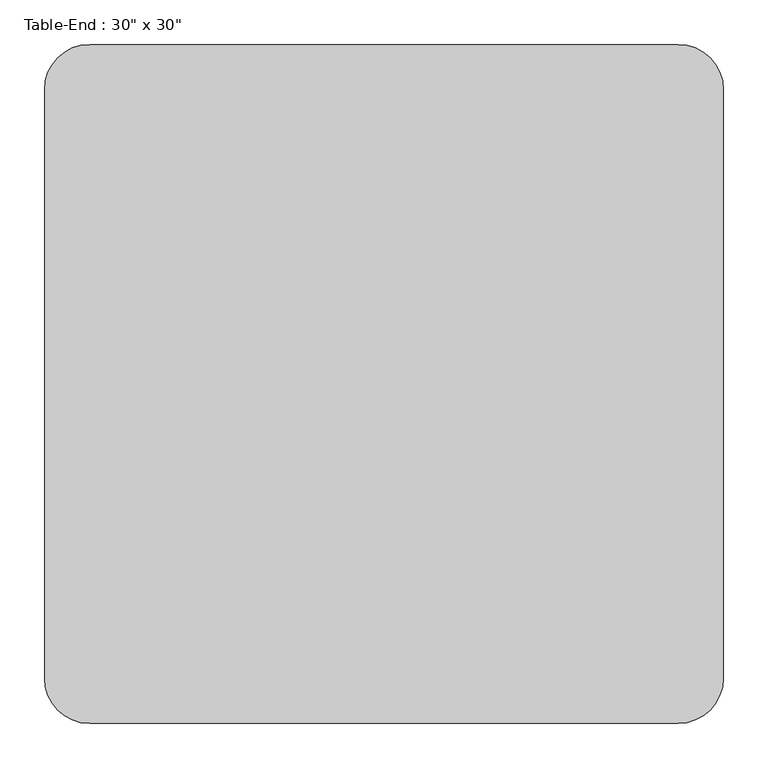
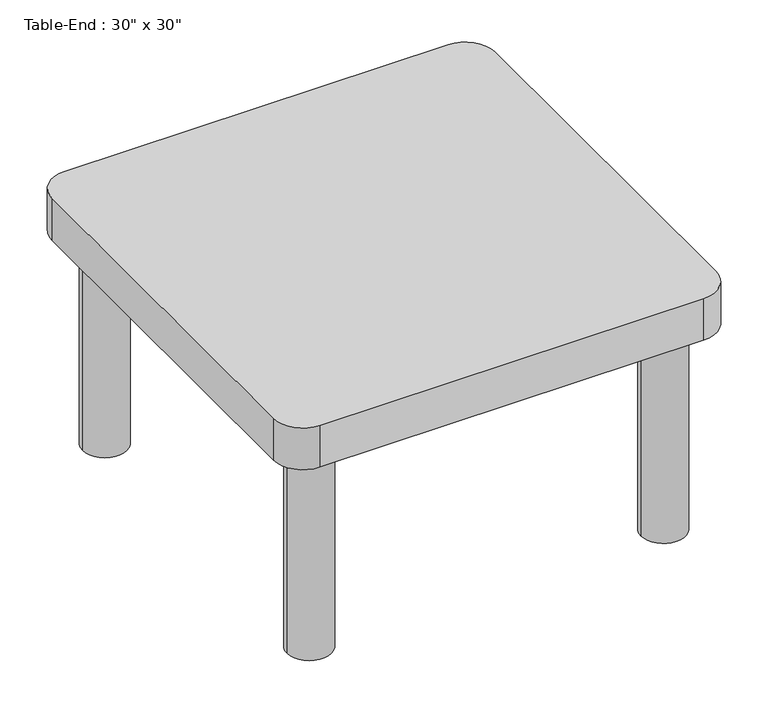
"""IFC4 building model written with IfcOpenShell, lengths in millimetres: furniture geometry."""

from ifc_helpers import new_model, si_unit, point, frame, frame_2d, origin, origin_with_axes, place, context, project, spatial, polyline, circle_curve, trimmed, segment, composite_curve, outline, extrude, source, transform, mapped, element, save


def furniture_db92a8cd(model_context):
    return source(origin(), model_context, "Body", "SweptSolid", [
        extrude(outline(composite_curve([segment(polyline([(714.9336303, -228.6), (54.5336303, -228.6)]), True, "CONTINUOUS"), segment(trimmed(circle_curve(frame_2d((54.5336303, -177.8)), 50.8), [point((54.5336303, -228.6))], [point((3.7336303, -177.8))], False, "CARTESIAN"), True, "CONTINUOUS"), segment(polyline([(3.7336303, -177.8), (3.7336303, 482.6)]), True, "CONTINUOUS"), segment(trimmed(circle_curve(frame_2d((54.5336303, 482.6)), 50.8), [point((3.7336303, 482.6))], [point((54.5336303, 533.4))], False, "CARTESIAN"), True, "CONTINUOUS"), segment(polyline([(54.5336303, 533.4), (714.9336303, 533.4)]), True, "CONTINUOUS"), segment(trimmed(circle_curve(frame_2d((714.9336303, 482.6)), 50.8), [point((714.9336303, 533.4))], [point((765.7336303, 482.6))], False, "CARTESIAN"), True, "CONTINUOUS"), segment(polyline([(765.7336303, 482.6), (765.7336303, -177.8)]), True, "CONTINUOUS"), segment(trimmed(circle_curve(frame_2d((714.9336303, -177.8)), 50.8), [point((765.7336303, -177.8))], [point((714.9336303, -228.6))], False, "CARTESIAN"), True, "CONTINUOUS")], self_intersect=False)), frame((0.0, 0.0, 381.0), z_axis=(0.0, 0.0, 1.0), x_axis=(1.0, 0.0, 0.0)), (0.0, 0.0, 1.0), 76.2),
        extrude(outline(composite_curve([segment(trimmed(circle_curve(frame_2d((79.9336303, 457.2)), 38.1), [point((41.8336303, 457.2))], [point((118.0336303, 457.2))], False, "CARTESIAN"), True, "CONTINUOUS"), segment(trimmed(circle_curve(frame_2d((79.9336303, 457.2)), 38.1), [point((118.0336303, 457.2))], [point((41.8336303, 457.2))], False, "CARTESIAN"), True, "CONTINUOUS")], self_intersect=False)), origin_with_axes(), (0.0, 0.0, 1.0), 381.0),
        extrude(outline(composite_curve([segment(trimmed(circle_curve(frame_2d((79.9336303, -152.4)), 38.1), [point((41.8336303, -152.4))], [point((118.0336303, -152.4))], False, "CARTESIAN"), True, "CONTINUOUS"), segment(trimmed(circle_curve(frame_2d((79.9336303, -152.4)), 38.1), [point((118.0336303, -152.4))], [point((41.8336303, -152.4))], False, "CARTESIAN"), True, "CONTINUOUS")], self_intersect=False)), origin_with_axes(), (0.0, 0.0, 1.0), 381.0),
        extrude(outline(composite_curve([segment(trimmed(circle_curve(frame_2d((689.5336303, -152.4)), 38.1), [point((651.4336303, -152.4))], [point((727.6336303, -152.4))], False, "CARTESIAN"), True, "CONTINUOUS"), segment(trimmed(circle_curve(frame_2d((689.5336303, -152.4)), 38.1), [point((727.6336303, -152.4))], [point((651.4336303, -152.4))], False, "CARTESIAN"), True, "CONTINUOUS")], self_intersect=False)), origin_with_axes(), (0.0, 0.0, 1.0), 381.0),
        extrude(outline(composite_curve([segment(trimmed(circle_curve(frame_2d((689.5336303, 457.2)), 38.1), [point((651.4336303, 457.2))], [point((727.6336303, 457.2))], False, "CARTESIAN"), True, "CONTINUOUS"), segment(trimmed(circle_curve(frame_2d((689.5336303, 457.2)), 38.1), [point((727.6336303, 457.2))], [point((651.4336303, 457.2))], False, "CARTESIAN"), True, "CONTINUOUS")], self_intersect=False)), origin_with_axes(), (0.0, 0.0, 1.0), 381.0),
    ])


if __name__ == "__main__":
    model = new_model("IFC4")
    model_context = context("Model", 3, world=origin())
    ifc_project = project(units=[si_unit("LENGTHUNIT", "METRE", prefix="MILLI")], contexts=[model_context])
    site = spatial("IfcSite", under=ifc_project)
    building = spatial("IfcBuilding", under=site)
    placement = place(None, origin())
    furniture_shape = furniture_db92a8cd(model_context)
    element("IfcFurniture", 1, ObjectType="Table-End : 30\" x 30\"", at=placement, inside=building, context=model_context, shape_type="MappedRepresentation", body=[
        mapped(furniture_shape, transform((0.0, 0.0, 0.0), x_axis=(1.0, 0.0, 0.0), y_axis=(0.0, 1.0, 0.0), z_axis=(0.0, 0.0, 1.0))),
    ])
    save(model, "model.ifc")

# Revit data of these elements
# Type "Table-End : 30\" x 30\""
#   Assembly Code = "E2020200"
#   Height = 1' - 6"
#   Length = 2' - 6"
#   Width = 2' - 6"
#   Base Material = Birch
#   Top Material = Laminate, Ivory, Matte
#   Default Elevation = 0
# Element 1 (IfcFurniture, "Table-End : 30\" x 30\"")
#   Materials on its faces: "Laminate, Ivory, Matte", "Birch"
# Materials
#   "Birch": class "Wood", colour RGB 224 178 126, transparency 0, Description = "Betula Alleghaniensis", Cost = 0
#   "Laminate, Ivory, Matte": class "Plastic", colour RGB 247 247 239, transparency 0, Description = "Plastic Laminate - Ivory, Matte", Cost = 0
